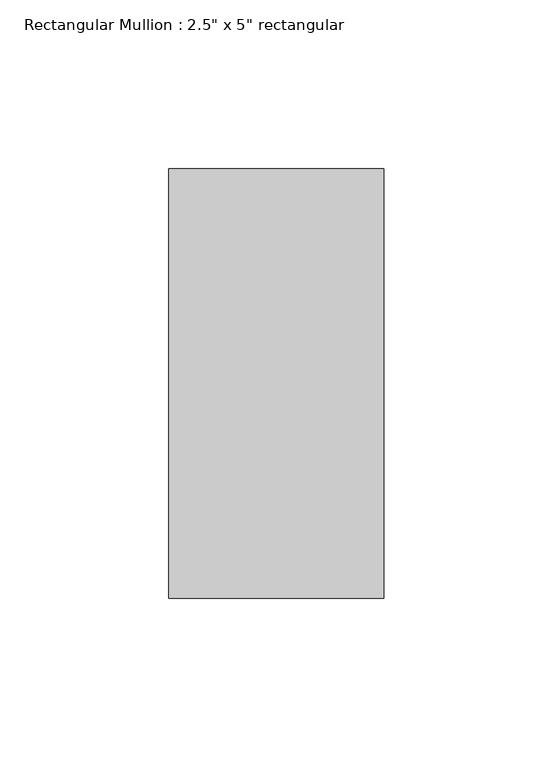
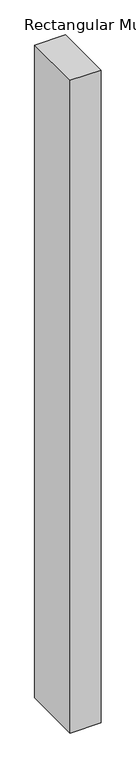
"""IFC4 building model written with IfcOpenShell, lengths in millimetres: member geometry."""

from ifc_helpers import new_model, si_unit, frame, origin, place, context, project, spatial, polyline, outline, extrude, source, transform, mapped, element, save


def member_8a84510b(model_context):
    return source(origin(), model_context, "Body", "SweptSolid", [
        extrude(outline(polyline([(0.0, 63.5), (0.0, -63.5), (-63.5, -63.5), (-63.5, 63.5), (0.0, 63.5)])), frame((0.0, 0.0, -1425.0105727), z_axis=(0.0, 0.0, 1.0), x_axis=(1.0, 0.0, 0.0)), (0.0, 0.0, 1.0), 1425.0105727),
    ])


if __name__ == "__main__":
    model = new_model("IFC4")
    model_context = context("Model", 3, world=origin())
    ifc_project = project(units=[si_unit("LENGTHUNIT", "METRE", prefix="MILLI")], contexts=[model_context])
    site = spatial("IfcSite", under=ifc_project)
    building = spatial("IfcBuilding", under=site)
    placement = place(None, origin())
    member_shape = member_8a84510b(model_context)
    element("IfcMember", 1, ObjectType="Rectangular Mullion : 2.5\" x 5\" rectangular", at=placement, inside=building, context=model_context, shape_type="MappedRepresentation", body=[
        mapped(member_shape, transform((0.0, 0.0, 0.0), x_axis=(1.0, 0.0, 0.0), y_axis=(0.0, 1.0, 0.0), z_axis=(0.0, 0.0, 1.0))),
    ])
    save(model, "model.ifc")

# Revit data of these elements
# Type "Rectangular Mullion : 2.5\" x 5\" rectangular"
#   built-in parameter 1007304 = 0.416667 (stored number, unit not read)
#   built-in parameter 1007301 = 0.104167 (stored number, unit not read)
#   built-in parameter 1007300 = 0.104167 (stored number, unit not read)
# Element 1 (IfcMember, "Rectangular Mullion : 2.5\" x 5\" rectangular")
#   Materials on its faces: "Aluminum"
# Materials
#   "Aluminum": class "Metal", colour RGB 247 247 247, transparency 0, Description = "Aluminum 6061", Cost = 0
